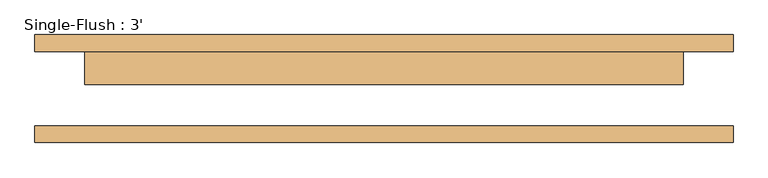
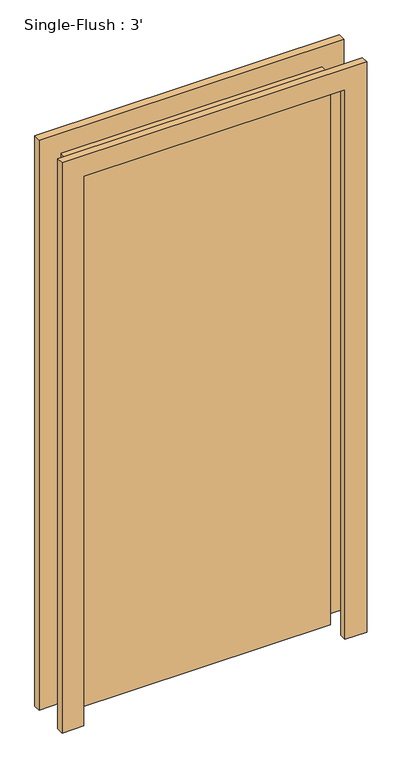
"""IFC4 building model written with IfcOpenShell, lengths in millimetres: door geometry, Single-Flush : 3'."""

from ifc_helpers import new_model, si_unit, frame, origin, origin_with_axes, place, context, project, spatial, polyline, outline, extrude, source, transform, mapped, element, save


def single_flush_3_17d80c48(model_context):
    return source(origin(), model_context, "Body", "SweptSolid", [
        extrude(outline(polyline([(2108.2, -533.4), (0.0, -533.4), (0.0, -457.2), (2032.0, -457.2), (2032.0, 457.2), (0.0, 457.2), (0.0, 533.4), (2108.2, 533.4), (2108.2, -533.4)])), frame((0.0, 57.15, 0.0), z_axis=(0.0, 1.0, 0.0), x_axis=(0.0, 0.0, 1.0)), (0.0, 0.0, 1.0), 25.4),
        extrude(outline(polyline([(2108.2, 533.4), (2108.2, -533.4), (0.0, -533.4), (0.0, -457.2), (2032.0, -457.2), (2032.0, 457.2), (0.0, 457.2), (0.0, 533.4), (2108.2, 533.4)])), frame((0.0, -82.55, 0.0), z_axis=(0.0, 1.0, 0.0), x_axis=(0.0, 0.0, 1.0)), (0.0, 0.0, 1.0), 25.4),
        extrude(outline(polyline([(457.2, 6.35), (-457.2, 6.35), (-457.2, 57.15), (457.2, 57.15), (457.2, 6.35)])), origin_with_axes(), (0.0, 0.0, 1.0), 2032.0),
    ])


if __name__ == "__main__":
    model = new_model("IFC4")
    model_context = context("Model", 3, world=origin())
    ifc_project = project(units=[si_unit("LENGTHUNIT", "METRE", prefix="MILLI")], contexts=[model_context])
    site = spatial("IfcSite", under=ifc_project)
    building = spatial("IfcBuilding", under=site)
    placement = place(None, origin())
    single_flush_3_shape = single_flush_3_17d80c48(model_context)
    element("IfcDoor", 1, ObjectType="Single-Flush : 3'", at=placement, inside=building, context=model_context, shape_type="MappedRepresentation", body=[
        mapped(single_flush_3_shape, transform((0.0, 0.0, 0.0), x_axis=(1.0, 0.0, 0.0), y_axis=(0.0, 1.0, 0.0), z_axis=(0.0, 0.0, 1.0))),
    ])
    save(model, "model.ifc")

# Revit data of these elements
# Type "Single-Flush : 3'"
#   Type Mark = "8"
#   Construction Type Id = "MDOOR"
#   Assembly Code = "C1020"
#   Analytic Construction = "Metal"
#   Thickness = 0' - 2"
#   Heat Transfer Coefficient (U) = 0.651978 BTU/(h·ft²·°F)
#   Height = 6' - 8"
#   Trim Projection Ext = 0' - 1"
#   Trim Projection Int = 0' - 1"
#   Trim Width = 0' - 3"
#   Width = 3' - 0"
#   Define Thermal Properties by = 1
#   Door Material = Door - Panel
#   Frame Material = Door - Frame
#   Visual Light Transmittance = 0
#   Solar Heat Gain Coefficient = 0
#   Function = (empty or 0)
#   Wall Closure = (empty or 0)
# Element 1 (IfcDoor, "Single-Flush : 3'")
#   Materials on its faces: "Door - Frame", "Door - Panel"
# Materials
#   "Door - Panel": class "Wood", colour RGB 210 159 95, transparency 0, Cost = 0
#   "Door - Frame": colour RGB 118 70 51, transparency 0, Cost = 0
